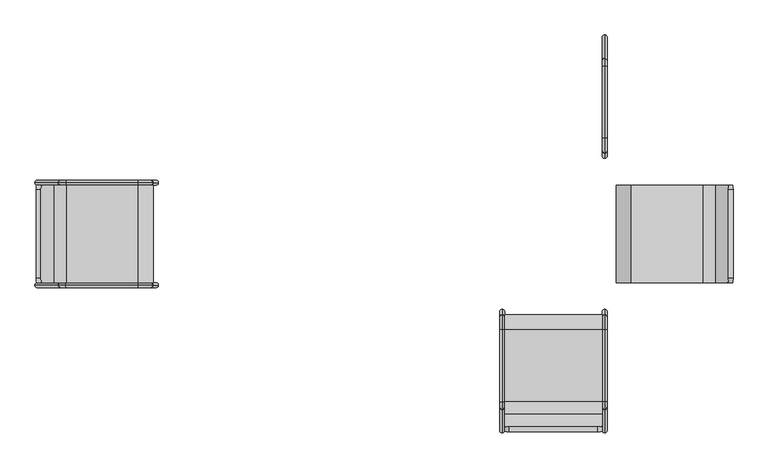
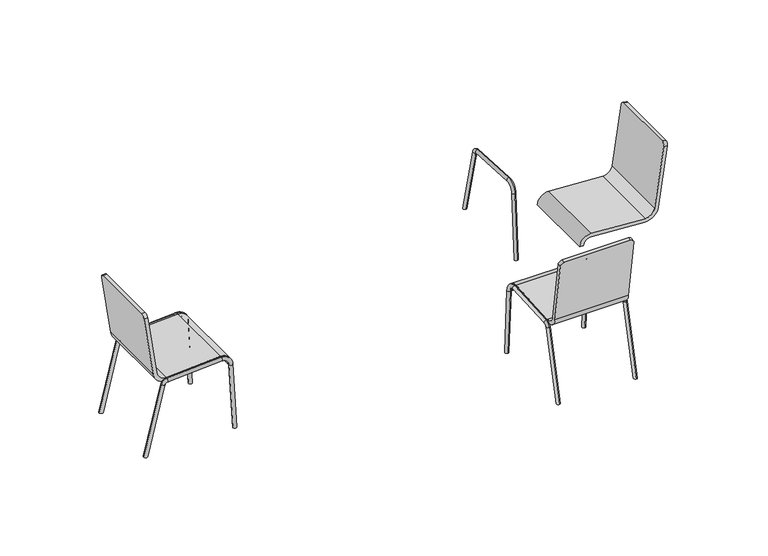
"""IFC4 building model written with IfcOpenShell, lengths in millimetres: furniture geometry."""

from ifc_helpers import new_model, si_unit, point, frame, origin, place, context, project, spatial, polyline, circle_curve, ellipse_curve, trimmed, source, transform, mapped, element, save
from ifc_brep_helpers import plane_surface, cylinder_surface, revolved_surface, advanced_brep


def furniture_b53a9923(model_context):
    return source(origin(), model_context, "Body", "AdvancedBrep", [
        advanced_brep(
        [(832.7255181, 202.5, 414.5657988), (885.0808804, 202.5, 457.0908917), (935.9370847, 202.5, 797.3777006), (955.717402, 202.5, 794.4215124), (904.8611977, 202.5, 454.1347035), (831.5636904, 202.5, 394.5995734), (535.5224482, 202.5, 411.8261096), (493.2663421, 202.5, 374.2173141), (473.3001167, 202.5, 375.3791418), (536.6842759, 202.5, 431.792335), (832.7255181, -202.5, 414.5657988), (536.6842759, -202.5, 431.792335), (473.3001167, -202.5, 375.3791418), (493.2663421, -202.5, 374.2173141), (535.5224482, -202.5, 411.8261096), (831.5636904, -202.5, 394.5995734), (904.8611977, -202.5, 454.1347035), (955.717402, -202.5, 794.4215124), (935.9370847, -202.5, 797.3777006), (885.0808804, -202.5, 457.0908917), (958.6735902, 182.5, 814.2018297), (958.6735902, -182.5, 814.2018297), (938.893273, 182.5, 817.1580179), (938.893273, -182.5, 817.1580179)],
        [
            (0, 1, circle_curve(frame((835.6300872, 202.5, 464.4813623), z_axis=(0.0, -1.0, 0.0), x_axis=(1.0, 0.0, 0.0)), 50.0)),
            (1, 2),
            (2, 3),
            (3, 4),
            (4, 5, circle_curve(frame((835.6300872, 202.5, 464.4813623), z_axis=(0.0, 1.0, 0.0), x_axis=(1.0, 0.0, 0.0)), 70.0)),
            (5, 6),
            (6, 7, circle_curve(frame((533.1987929, 202.5, 371.8936588), z_axis=(0.0, -1.0, 0.0), x_axis=(1.0, 0.0, 0.0)), 40.0)),
            (7, 8),
            (8, 9, circle_curve(frame((533.1987929, 202.5, 371.8936588), z_axis=(0.0, 1.0, 0.0), x_axis=(1.0, 0.0, 0.0)), 60.0)),
            (9, 0),
            (10, 11),
            (11, 12, circle_curve(frame((533.1987929, -202.5, 371.8936588), z_axis=(0.0, -1.0, 0.0), x_axis=(1.0, 0.0, 0.0)), 60.0)),
            (12, 13),
            (13, 14, circle_curve(frame((533.1987929, -202.5, 371.8936588), z_axis=(0.0, 1.0, 0.0), x_axis=(1.0, 0.0, 0.0)), 40.0)),
            (14, 15),
            (15, 16, circle_curve(frame((835.6300872, -202.5, 464.4813623), z_axis=(0.0, -1.0, 0.0), x_axis=(1.0, 0.0, 0.0)), 70.0)),
            (16, 17),
            (17, 18),
            (18, 19),
            (19, 10, circle_curve(frame((835.6300872, -202.5, 464.4813623), z_axis=(0.0, 1.0, 0.0), x_axis=(1.0, 0.0, 0.0)), 50.0)),
            (9, 11),
            (10, 0),
            (8, 12),
            (7, 13),
            (6, 14),
            (5, 15),
            (4, 16),
            (3, 20, circle_curve(frame((955.717402, 182.5, 794.4215124), z_axis=(0.9890158633619166, 0.0, -0.14780941112961252), x_axis=(0.0, -1.0, 0.0)), 20.0)),
            (20, 21),
            (21, 17, circle_curve(frame((955.717402, -182.5, 794.4215124), z_axis=(0.9890158633619166, 0.0, -0.14780941112961252), x_axis=(0.0, 1.0, 0.0)), 20.0)),
            (20, 22),
            (22, 23),
            (23, 21),
            (18, 23, circle_curve(frame((935.9370847, -182.5, 797.3777006), z_axis=(-0.9890158633619166, 0.0, 0.14780941112961252), x_axis=(0.0, 1.0, 0.0)), 20.0)),
            (22, 2, circle_curve(frame((935.9370847, 182.5, 797.3777006), z_axis=(-0.9890158633619166, 0.0, 0.14780941112961252), x_axis=(0.0, -1.0, 0.0)), 20.0)),
            (1, 19),
        ],
        [
            plane_surface(frame((538.9293412, 202.5, 431.6616954), z_axis=(0.0, 1.0000000000000002, 0.0), x_axis=(-0.9983112697039764, 0.0, 0.05809138302738736))),
            plane_surface(frame((538.9293412, -202.5, 431.6616954), z_axis=(0.0, -1.0000000000000002, 0.0), x_axis=(0.9983112697039764, 0.0, -0.05809138302738736))),
            plane_surface(frame((832.7255181, 202.5, 414.5657988), z_axis=(0.05809138302738736, 0.0, 0.9983112697039764), x_axis=(0.0, -1.0, 0.0))),
            cylinder_surface(frame((533.1987929, -202.5, 371.8936588), z_axis=(0.0, 1.0, 0.0), x_axis=(1.0, 0.0, 0.0)), 60.0),
            plane_surface(frame((473.3001167, 202.5, 375.3791418), z_axis=(-0.058091383027390926, 0.0, -0.9983112697039762), x_axis=(0.0, -1.0, 0.0))),
            revolved_surface(polyline([(573.1987929, -202.5, 371.8936588), (573.1987929, 202.5, 371.8936588)]), (533.1987929, -202.5, 371.8936588), (0.0, -1.0, 0.0)),
            plane_surface(frame((535.5224482, 202.5, 411.8261096), z_axis=(-0.05809138302738756, 0.0, -0.9983112697039763), x_axis=(0.0, -1.0, 0.0))),
            cylinder_surface(frame((835.6300872, -202.5, 464.4813623), z_axis=(0.0, 1.0, 0.0), x_axis=(1.0, 0.0, 0.0)), 70.0),
            plane_surface(frame((904.8611977, 202.5, 454.1347035), z_axis=(0.9890158633619166, 0.0, -0.1478094111296125), x_axis=(0.0, -1.0, 0.0))),
            plane_surface(frame((958.6735902, 202.5, 814.2018297), z_axis=(0.14780941112961524, 0.0, 0.9890158633619162), x_axis=(0.0, -1.0, 0.0))),
            plane_surface(frame((938.893273, 202.5, 817.1580179), z_axis=(-0.9890158633619166, 0.0, 0.14780941112961254), x_axis=(0.0, -1.0, 0.0))),
            revolved_surface(polyline([(885.6300872, -202.5, 464.4813623), (885.6300872, 202.5, 464.4813623)]), (835.6300872, -202.5, 464.4813623), (0.0, -1.0, 0.0)),
            cylinder_surface(frame((935.9370847, -182.5, 797.3777006), z_axis=(-0.9890158633619166, 0.0, 0.14780941112961252), x_axis=(0.0, 1.0, 0.0)), 20.0),
            cylinder_surface(frame((935.9370847, 182.5, 797.3777006), z_axis=(-0.9890158633619166, 0.0, 0.14780941112961252), x_axis=(0.0, -1.0, 0.0)), 20.0),
        ],
        [
            (0, [[1, 2, 3, 4, 5, 6, 7, 8, 9, 10]]),
            (1, [[11, 12, 13, 14, 15, 16, 17, 18, 19, 20]]),
            (2, [[21, -11, 22, -10]]),
            (3, [[23, -12, -21, -9]]),
            (4, [[24, -13, -23, -8]]),
            (5, [[25, -14, -24, -7]]),
            (6, [[26, -15, -25, -6]]),
            (7, [[27, -16, -26, -5]]),
            (8, [[-4, 28, 29, 30, -17, -27]]),
            (9, [[31, 32, 33, -29]]),
            (10, [[-19, 34, -32, 35, -2, 36]]),
            (11, [[-22, -20, -36, -1]]),
            (12, [[-30, -33, -34, -18]]),
            (13, [[-35, -31, -28, -3]]),
        ],
    ),
        advanced_brep(
        [(-1916.2585347, 212.5797007, 0.0), (-1936.8708073, 212.5797007, 0.0), (-1434.6031938, 222.5797007, 0.0), (-1434.6031938, 202.5797007, 0.0), (-1444.6201096, 212.5797007, 0.0), (-1820.7368981, 212.5797007, 383.1163586), (-1840.1428126, 212.5797007, 387.9547965), (-1807.053833, 212.5797007, 394.4621992), (-1808.2156606, 212.5797007, 414.4284246), (-1508.6517901, 212.5797007, 411.8261096), (-1509.8136178, 212.5797007, 431.792335), (-1466.395684, 212.5797007, 374.2173141), (-1446.4294586, 212.5797007, 375.3791418), (-1424.6200811, 212.5797007, 0.5809138)],
        [
            (0, 1, ellipse_curve(frame((-1926.564671, 212.5797007, 0.0), z_axis=(0.0, 0.0, -1.0), x_axis=(-1.0, 0.0, 0.0)), 10.3061363, 10.0)),
            (1, 0, ellipse_curve(frame((-1926.564671, 212.5797007, 0.0), z_axis=(0.0, 0.0, -1.0), x_axis=(-1.0, 0.0, 0.0)), 10.3061363, 10.0)),
            (2, 3),
            (3, 4, ellipse_curve(frame((-1434.6031938, 212.5797007, 0.0), z_axis=(0.0, 0.0, -1.0), x_axis=(-1.0, 0.0, 0.0)), 10.0169159, 10.0)),
            (4, 2, ellipse_curve(frame((-1434.6031938, 212.5797007, 0.0), z_axis=(0.0, 0.0, -1.0), x_axis=(-1.0, 0.0, 0.0)), 10.0169159, 10.0)),
            (5, 6, circle_curve(frame((-1830.4398554, 212.5797007, 385.5355776), z_axis=(-0.24192189559966623, 0.0, -0.9702957262759968), x_axis=(-0.9702957262759968, 0.0, 0.24192189559966623)), 10.0)),
            (6, 1),
            (0, 5),
            (6, 5, circle_curve(frame((-1830.4398554, 212.5797007, 385.5355776), z_axis=(-0.24192189559966623, 0.0, -0.9702957262759968), x_axis=(-0.9702957262759968, 0.0, 0.24192189559966623)), 10.0)),
            (5, 7, circle_curve(frame((-1806.1824622, 212.5797007, 379.4875302), z_axis=(0.0, 1.0, 0.0), x_axis=(-0.9702957262759969, 0.0, 0.2419218955996659)), 15.0)),
            (7, 8, circle_curve(frame((-1807.6347468, 212.5797007, 404.4453119), z_axis=(-0.998311269703977, 0.0, -0.058091383027376764), x_axis=(-0.058091383027376764, 0.0, 0.998311269703977)), 10.0)),
            (8, 6, circle_curve(frame((-1806.1824622, 212.5797007, 379.4875302), z_axis=(0.0, -1.0, 0.0), x_axis=(-0.9702957262759969, 0.0, 0.2419218955996659)), 35.0)),
            (8, 7, circle_curve(frame((-1807.6347468, 212.5797007, 404.4453119), z_axis=(-0.9983112697039765, 0.0, -0.05809138302738498), x_axis=(-0.05809138302738498, 0.0, 0.9983112697039765)), 10.0)),
            (7, 9),
            (9, 10, circle_curve(frame((-1509.232704, 212.5797007, 421.8092223), z_axis=(-0.9983112697039764, 0.0, -0.058091383027386895), x_axis=(-0.058091383027386895, 0.0, 0.9983112697039764)), 10.0)),
            (10, 8),
            (10, 9, circle_curve(frame((-1509.232704, 212.5797007, 421.8092223), z_axis=(-0.9983112697039764, 0.0, -0.058091383027386895), x_axis=(-0.058091383027386895, 0.0, 0.9983112697039764)), 10.0)),
            (9, 11, circle_curve(frame((-1506.3281348, 212.5797007, 371.8936588), z_axis=(0.0, 1.0, 0.0), x_axis=(-0.05809138302738633, 0.0, 0.9983112697039764)), 40.0)),
            (11, 12, circle_curve(frame((-1456.4125713, 212.5797007, 374.7982279), z_axis=(-0.058091383027391474, 0.0, 0.9983112697039761), x_axis=(0.9983112697039761, 0.0, 0.058091383027391474)), 10.0)),
            (12, 10, circle_curve(frame((-1506.3281348, 212.5797007, 371.8936588), z_axis=(0.0, -1.0, 0.0), x_axis=(-0.05809138302738633, 0.0, 0.9983112697039764)), 60.0)),
            (12, 11, circle_curve(frame((-1456.4125713, 212.5797007, 374.7982279), z_axis=(-0.05809138302739081, 0.0, 0.9983112697039762), x_axis=(0.9983112697039762, 0.0, 0.05809138302739081)), 10.0)),
            (2, 13, circle_curve(frame((-1434.6031938, 212.5797007, 0.0), z_axis=(0.058091383027392335, 0.0, -0.9983112697039761), x_axis=(0.9983112697039761, 0.0, 0.058091383027392335)), 10.0)),
            (13, 3, circle_curve(frame((-1434.6031938, 212.5797007, 0.0), z_axis=(0.058091383027392335, 0.0, -0.9983112697039761), x_axis=(0.9983112697039761, 0.0, 0.058091383027392335)), 10.0)),
            (11, 4),
            (13, 12),
        ],
        [
            plane_surface(frame((-1962.0110531, 250.0, 0.0), z_axis=(0.0, 0.0, -1.0), x_axis=(0.0, -1.0, 0.0))),
            cylinder_surface(frame((-1929.1748213, 212.5797007, -10.4687411), z_axis=(-0.24192189559966623, 0.0, -0.9702957262759968), x_axis=(-0.9702957262759968, 0.0, 0.24192189559966623)), 10.0),
            revolved_surface(trimmed(ellipse_curve(frame((-1830.4398554, 212.5797007, 385.5355776), z_axis=(-0.2419218955996659, 0.0, -0.9702957262759969), x_axis=(-0.9702957262759969, 0.0, 0.2419218955996659)), 10.0, 10.0), [point((-1820.7368981, 212.5797007, 383.1163586))], [point((-1840.1428126, 212.5797007, 387.9547965))], True, "CARTESIAN"), (-1806.1824622, 192.5797007, 379.4875302), (0.0, 1.0, 0.0)),
            revolved_surface(trimmed(ellipse_curve(frame((-1830.4398554, 212.5797007, 385.5355776), z_axis=(-0.2419218955996659, 0.0, -0.9702957262759969), x_axis=(-0.9702957262759969, 0.0, 0.2419218955996659)), 10.0, 10.0), [point((-1840.1428126, 212.5797007, 387.9547965))], [point((-1820.7368981, 212.5797007, 383.1163586))], True, "CARTESIAN"), (-1806.1824622, 192.5797007, 379.4875302), (0.0, 1.0, 0.0)),
            cylinder_surface(frame((-1807.6347468, 212.5797007, 404.4453119), z_axis=(-0.9983112697039764, 0.0, -0.058091383027386895), x_axis=(-0.058091383027386895, 0.0, 0.9983112697039764)), 10.0),
            revolved_surface(trimmed(ellipse_curve(frame((-1509.232704, 212.5797007, 421.8092223), z_axis=(-0.9983112697039764, 0.0, -0.05809138302738631), x_axis=(-0.05809138302738631, 0.0, 0.9983112697039764)), 10.0, 10.0), [point((-1508.6517901, 212.5797007, 411.8261096))], [point((-1509.8136178, 212.5797007, 431.792335))], True, "CARTESIAN"), (-1506.3281348, 192.5797007, 371.8936588), (0.0, 1.0, 0.0)),
            revolved_surface(trimmed(ellipse_curve(frame((-1509.232704, 212.5797007, 421.8092223), z_axis=(-0.9983112697039764, 0.0, -0.05809138302738631), x_axis=(-0.05809138302738631, 0.0, 0.9983112697039764)), 10.0, 10.0), [point((-1509.8136178, 212.5797007, 431.792335))], [point((-1508.6517901, 212.5797007, 411.8261096))], True, "CARTESIAN"), (-1506.3281348, 192.5797007, 371.8936588), (0.0, 1.0, 0.0)),
            plane_surface(frame((-1434.6031938, 192.5797007, 0.0), z_axis=(0.058091383027392335, 0.0, -0.9983112697039761), x_axis=(0.0, 1.0, 0.0))),
            cylinder_surface(frame((-1456.4125713, 212.5797007, 374.7982279), z_axis=(-0.058091383027392335, 0.0, 0.9983112697039761), x_axis=(0.9983112697039761, 0.0, 0.058091383027392335)), 10.0),
        ],
        [
            (0, [[1, 2]]),
            (0, [[3, 4, 5]]),
            (1, [[6, 7, -1, 8]]),
            (1, [[9, -8, -2, -7]]),
            (2, [[-6, 10, 11, 12]]),
            (3, [[-9, -12, 13, -10]]),
            (4, [[-11, 14, 15, 16]]),
            (4, [[-13, -16, 17, -14]]),
            (5, [[-15, 18, 19, 20]]),
            (6, [[-17, -20, 21, -18]]),
            (7, [[22, 23, -3]]),
            (8, [[-19, 24, -4, -23, 25]]),
            (8, [[-21, -25, -22, -5, -24]]),
        ],
    ),
        advanced_brep(
        [(-1434.6031938, -202.5797007, 0.0), (-1424.6200811, -212.5797007, 0.5809138), (-1434.6031938, -222.5797007, 0.0), (-1820.7368981, -212.5797007, 383.1163586), (-1840.1428126, -212.5797007, 387.9547965), (-1936.8708073, -212.5797007, 0.0), (-1916.2585347, -212.5797007, 0.0), (-1444.6201096, -212.5797007, 0.0), (-1808.2156606, -212.5797007, 414.4284246), (-1807.053833, -212.5797007, 394.4621992), (-1508.6517901, -212.5797007, 411.8261096), (-1509.8136178, -212.5797007, 431.792335), (-1466.395684, -212.5797007, 374.2173141), (-1446.4294586, -212.5797007, 375.3791418)],
        [
            (0, 1, circle_curve(frame((-1434.6031938, -212.5797007, 0.0), z_axis=(0.058091383027392335, 0.0, -0.9983112697039761), x_axis=(0.9983112697039761, 0.0, 0.058091383027392335)), 10.0)),
            (1, 2, circle_curve(frame((-1434.6031938, -212.5797007, 0.0), z_axis=(0.058091383027392335, 0.0, -0.9983112697039761), x_axis=(0.9983112697039761, 0.0, 0.058091383027392335)), 10.0)),
            (2, 0),
            (3, 4, circle_curve(frame((-1830.4398554, -212.5797007, 385.5355776), z_axis=(-0.24192189559966623, 0.0, -0.9702957262759968), x_axis=(-0.9702957262759968, 0.0, 0.24192189559966623)), 10.0)),
            (4, 5),
            (5, 6, ellipse_curve(frame((-1926.564671, -212.5797007, 0.0), z_axis=(0.0, 0.0, 1.0), x_axis=(-1.0, 0.0, 0.0)), 10.3061363, 10.0)),
            (6, 3),
            (4, 3, circle_curve(frame((-1830.4398554, -212.5797007, 385.5355776), z_axis=(-0.24192189559966623, 0.0, -0.9702957262759968), x_axis=(-0.9702957262759968, 0.0, 0.24192189559966623)), 10.0)),
            (6, 5, ellipse_curve(frame((-1926.564671, -212.5797007, 0.0), z_axis=(0.0, 0.0, 1.0), x_axis=(-1.0, 0.0, 0.0)), 10.3061363, 10.0)),
            (2, 7, ellipse_curve(frame((-1434.6031938, -212.5797007, 0.0), z_axis=(0.0, 0.0, -1.0), x_axis=(-1.0, 0.0, 0.0)), 10.0169159, 10.0)),
            (7, 0, ellipse_curve(frame((-1434.6031938, -212.5797007, 0.0), z_axis=(0.0, 0.0, -1.0), x_axis=(-1.0, 0.0, 0.0)), 10.0169159, 10.0)),
            (8, 9, circle_curve(frame((-1807.6347468, -212.5797007, 404.4453119), z_axis=(0.9983112697039764, 0.0, 0.058091383027386895), x_axis=(-0.058091383027386895, 0.0, 0.9983112697039764)), 10.0)),
            (9, 10),
            (10, 11, circle_curve(frame((-1509.232704, -212.5797007, 421.8092223), z_axis=(-0.9983112697039764, 0.0, -0.058091383027386895), x_axis=(-0.058091383027386895, 0.0, 0.9983112697039764)), 10.0)),
            (11, 8),
            (9, 8, circle_curve(frame((-1807.6347468, -212.5797007, 404.4453119), z_axis=(0.9983112697039764, 0.0, 0.058091383027386895), x_axis=(-0.058091383027386895, 0.0, 0.9983112697039764)), 10.0)),
            (11, 10, circle_curve(frame((-1509.232704, -212.5797007, 421.8092223), z_axis=(-0.9983112697039764, 0.0, -0.058091383027386895), x_axis=(-0.058091383027386895, 0.0, 0.9983112697039764)), 10.0)),
            (10, 12, circle_curve(frame((-1506.3281348, -212.5797007, 371.8936588), z_axis=(0.0, 1.0, 0.0), x_axis=(-0.05809138302738633, 0.0, 0.9983112697039764)), 40.0)),
            (12, 13, circle_curve(frame((-1456.4125713, -212.5797007, 374.7982279), z_axis=(-0.058091383027391474, 0.0, 0.9983112697039761), x_axis=(0.9983112697039761, 0.0, 0.058091383027391474)), 10.0)),
            (13, 11, circle_curve(frame((-1506.3281348, -212.5797007, 371.8936588), z_axis=(0.0, -1.0, 0.0), x_axis=(-0.05809138302738633, 0.0, 0.9983112697039764)), 60.0)),
            (13, 12, circle_curve(frame((-1456.4125713, -212.5797007, 374.7982279), z_axis=(-0.05809138302739081, 0.0, 0.9983112697039762), x_axis=(0.9983112697039762, 0.0, 0.05809138302739081)), 10.0)),
            (12, 7),
            (1, 13),
            (3, 9, circle_curve(frame((-1806.1824622, -212.5797007, 379.4875302), z_axis=(0.0, 1.0, 0.0), x_axis=(-0.9702957262759969, 0.0, 0.2419218955996659)), 15.0)),
            (8, 4, circle_curve(frame((-1806.1824622, -212.5797007, 379.4875302), z_axis=(0.0, -1.0, 0.0), x_axis=(-0.9702957262759969, 0.0, 0.2419218955996659)), 35.0)),
        ],
        [
            plane_surface(frame((-1434.6031938, -192.5797007, 0.0), z_axis=(0.058091383027392335, 0.0, -0.9983112697039761), x_axis=(0.0, -1.0, 0.0))),
            cylinder_surface(frame((-1929.1748213, -212.5797007, -10.4687411), z_axis=(-0.24192189559966623, 0.0, -0.9702957262759968), x_axis=(-0.9702957262759968, 0.0, 0.24192189559966623)), 10.0),
            plane_surface(frame((-1962.0110531, 250.0, 0.0), z_axis=(0.0, 0.0, -1.0), x_axis=(0.0, -1.0, 0.0))),
            cylinder_surface(frame((-1807.6347468, -212.5797007, 404.4453119), z_axis=(-0.9983112697039764, 0.0, -0.058091383027386895), x_axis=(-0.058091383027386895, 0.0, 0.9983112697039764)), 10.0),
            revolved_surface(trimmed(ellipse_curve(frame((-1509.232704, -212.5797007, 421.8092223), z_axis=(-0.9983112697039764, 0.0, -0.05809138302738631), x_axis=(-0.05809138302738631, 0.0, 0.9983112697039764)), 10.0, 10.0), [point((-1508.6517901, -212.5797007, 411.8261096))], [point((-1509.8136178, -212.5797007, 431.792335))], True, "CARTESIAN"), (-1506.3281348, -192.5797007, 371.8936588), (0.0, 1.0, 0.0)),
            revolved_surface(trimmed(ellipse_curve(frame((-1509.232704, -212.5797007, 421.8092223), z_axis=(-0.9983112697039764, 0.0, -0.05809138302738631), x_axis=(-0.05809138302738631, 0.0, 0.9983112697039764)), 10.0, 10.0), [point((-1509.8136178, -212.5797007, 431.792335))], [point((-1508.6517901, -212.5797007, 411.8261096))], True, "CARTESIAN"), (-1506.3281348, -192.5797007, 371.8936588), (0.0, 1.0, 0.0)),
            cylinder_surface(frame((-1456.4125713, -212.5797007, 374.7982279), z_axis=(-0.058091383027392335, 0.0, 0.9983112697039761), x_axis=(0.9983112697039761, 0.0, 0.058091383027392335)), 10.0),
            revolved_surface(trimmed(ellipse_curve(frame((-1830.4398554, -212.5797007, 385.5355776), z_axis=(-0.2419218955996659, 0.0, -0.9702957262759969), x_axis=(-0.9702957262759969, 0.0, 0.2419218955996659)), 10.0, 10.0), [point((-1820.7368981, -212.5797007, 383.1163586))], [point((-1840.1428126, -212.5797007, 387.9547965))], True, "CARTESIAN"), (-1806.1824622, -192.5797007, 379.4875302), (0.0, 1.0, 0.0)),
            revolved_surface(trimmed(ellipse_curve(frame((-1830.4398554, -212.5797007, 385.5355776), z_axis=(-0.2419218955996659, 0.0, -0.9702957262759969), x_axis=(-0.9702957262759969, 0.0, 0.2419218955996659)), 10.0, 10.0), [point((-1840.1428126, -212.5797007, 387.9547965))], [point((-1820.7368981, -212.5797007, 383.1163586))], True, "CARTESIAN"), (-1806.1824622, -192.5797007, 379.4875302), (0.0, 1.0, 0.0)),
        ],
        [
            (0, [[1, 2, 3]]),
            (1, [[4, 5, 6, 7]]),
            (1, [[8, -7, 9, -5]]),
            (2, [[-3, 10, 11]]),
            (2, [[-6, -9]]),
            (3, [[12, 13, 14, 15]]),
            (3, [[16, -15, 17, -13]]),
            (4, [[-14, 18, 19, 20]]),
            (5, [[-17, -20, 21, -18]]),
            (6, [[-19, 22, -10, -2, 23]]),
            (6, [[-21, -23, -1, -11, -22]]),
            (7, [[-4, 24, -12, 25]]),
            (8, [[-8, -25, -16, -24]]),
        ],
    ),
        advanced_brep(
        [(-1805.85486, 202.5, 414.5657988), (-1509.8136178, 202.5, 431.792335), (-1446.4294586, 202.5, 375.3791418), (-1466.395684, 202.5, 374.2173141), (-1508.6517901, 202.5, 411.8261096), (-1804.6930323, 202.5, 394.5995734), (-1877.9905396, 202.5, 454.1347035), (-1928.8467439, 202.5, 794.4215124), (-1909.0664267, 202.5, 797.3777006), (-1858.2102223, 202.5, 457.0908917), (-1805.85486, -202.5, 414.5657988), (-1858.2102223, -202.5, 457.0908917), (-1909.0664267, -202.5, 797.3777006), (-1928.8467439, -202.5, 794.4215124), (-1877.9905396, -202.5, 454.1347035), (-1804.6930323, -202.5, 394.5995734), (-1508.6517901, -202.5, 411.8261096), (-1466.395684, -202.5, 374.2173141), (-1446.4294586, -202.5, 375.3791418), (-1509.8136178, -202.5, 431.792335), (-1931.8029322, -182.5, 814.2018297), (-1931.8029322, 182.5, 814.2018297), (-1912.0226149, -182.5, 817.1580179), (-1912.0226149, 182.5, 817.1580179)],
        [
            (0, 1),
            (1, 2, circle_curve(frame((-1506.3281348, 202.5, 371.8936588), z_axis=(0.0, 1.0, 0.0), x_axis=(-1.0, 0.0, 0.0)), 60.0)),
            (2, 3),
            (3, 4, circle_curve(frame((-1506.3281348, 202.5, 371.8936588), z_axis=(0.0, -1.0, 0.0), x_axis=(-1.0, 0.0, 0.0)), 40.0)),
            (4, 5),
            (5, 6, circle_curve(frame((-1808.7594292, 202.5, 464.4813623), z_axis=(0.0, 1.0, 0.0), x_axis=(-1.0, 0.0, 0.0)), 70.0)),
            (6, 7),
            (7, 8),
            (8, 9),
            (9, 0, circle_curve(frame((-1808.7594292, 202.5, 464.4813623), z_axis=(0.0, -1.0, 0.0), x_axis=(-1.0, 0.0, 0.0)), 50.0)),
            (10, 11, circle_curve(frame((-1808.7594292, -202.5, 464.4813623), z_axis=(0.0, 1.0, 0.0), x_axis=(-1.0, 0.0, 0.0)), 50.0)),
            (11, 12),
            (12, 13),
            (13, 14),
            (14, 15, circle_curve(frame((-1808.7594292, -202.5, 464.4813623), z_axis=(0.0, -1.0, 0.0), x_axis=(-1.0, 0.0, 0.0)), 70.0)),
            (15, 16),
            (16, 17, circle_curve(frame((-1506.3281348, -202.5, 371.8936588), z_axis=(0.0, 1.0, 0.0), x_axis=(-1.0, 0.0, 0.0)), 40.0)),
            (17, 18),
            (18, 19, circle_curve(frame((-1506.3281348, -202.5, 371.8936588), z_axis=(0.0, -1.0, 0.0), x_axis=(-1.0, 0.0, 0.0)), 60.0)),
            (19, 10),
            (0, 10),
            (19, 1),
            (18, 2),
            (17, 3),
            (16, 4),
            (15, 5),
            (14, 6),
            (13, 20, circle_curve(frame((-1928.8467439, -182.5, 794.4215124), z_axis=(-0.9890158633619166, 0.0, -0.14780941112961252), x_axis=(0.0, 1.0, 0.0)), 20.0)),
            (20, 21),
            (21, 7, circle_curve(frame((-1928.8467439, 182.5, 794.4215124), z_axis=(-0.9890158633619166, 0.0, -0.14780941112961252), x_axis=(0.0, -1.0, 0.0)), 20.0)),
            (20, 22),
            (22, 23),
            (23, 21),
            (11, 9),
            (8, 23, circle_curve(frame((-1909.0664267, 182.5, 797.3777006), z_axis=(0.9890158633619166, 0.0, 0.14780941112961252), x_axis=(0.0, -1.0, 0.0)), 20.0)),
            (22, 12, circle_curve(frame((-1909.0664267, -182.5, 797.3777006), z_axis=(0.9890158633619166, 0.0, 0.14780941112961252), x_axis=(0.0, 1.0, 0.0)), 20.0)),
        ],
        [
            plane_surface(frame((-1512.0586831, 202.5, 431.6616954), z_axis=(0.0, 1.0000000000000002, 0.0), x_axis=(0.9983112697039764, 0.0, 0.05809138302738736))),
            plane_surface(frame((-1512.0586831, -202.5, 431.6616954), z_axis=(0.0, -1.0000000000000002, 0.0), x_axis=(-0.9983112697039764, 0.0, -0.05809138302738736))),
            plane_surface(frame((-1805.85486, 202.5, 414.5657988), z_axis=(-0.05809138302738736, 0.0, 0.9983112697039764), x_axis=(0.0, -1.0, 0.0))),
            cylinder_surface(frame((-1506.3281348, -202.5, 371.8936588), z_axis=(0.0, 1.0, 0.0), x_axis=(-1.0, 0.0, 0.0)), 60.0),
            plane_surface(frame((-1446.4294586, 202.5, 375.3791418), z_axis=(0.058091383027390926, 0.0, -0.9983112697039762), x_axis=(0.0, -1.0, 0.0))),
            revolved_surface(polyline([(-1546.3281348, -202.5, 371.8936588), (-1546.3281348, 202.5, 371.8936588)]), (-1506.3281348, -202.5, 371.8936588), (0.0, -1.0, 0.0)),
            plane_surface(frame((-1508.6517901, 202.5, 411.8261096), z_axis=(0.05809138302738756, 0.0, -0.9983112697039763), x_axis=(0.0, -1.0, 0.0))),
            cylinder_surface(frame((-1808.7594292, -202.5, 464.4813623), z_axis=(0.0, 1.0, 0.0), x_axis=(-1.0, 0.0, 0.0)), 70.0),
            plane_surface(frame((-1877.9905396, 202.5, 454.1347035), z_axis=(-0.9890158633619166, 0.0, -0.1478094111296125), x_axis=(0.0, -1.0, 0.0))),
            plane_surface(frame((-1931.8029322, 202.5, 814.2018297), z_axis=(-0.14780941112961524, 0.0, 0.9890158633619162), x_axis=(0.0, -1.0, 0.0))),
            plane_surface(frame((-1912.0226149, 202.5, 817.1580179), z_axis=(0.9890158633619166, 0.0, 0.14780941112961254), x_axis=(0.0, -1.0, 0.0))),
            revolved_surface(polyline([(-1858.7594292, -202.5, 464.4813623), (-1858.7594292, 202.5, 464.4813623)]), (-1808.7594292, -202.5, 464.4813623), (0.0, -1.0, 0.0)),
            cylinder_surface(frame((-1909.0664267, -182.5, 797.3777006), z_axis=(0.9890158633619166, 0.0, 0.14780941112961252), x_axis=(0.0, 1.0, 0.0)), 20.0),
            cylinder_surface(frame((-1909.0664267, 182.5, 797.3777006), z_axis=(0.9890158633619166, 0.0, 0.14780941112961252), x_axis=(0.0, -1.0, 0.0)), 20.0),
        ],
        [
            (0, [[1, 2, 3, 4, 5, 6, 7, 8, 9, 10]]),
            (1, [[11, 12, 13, 14, 15, 16, 17, 18, 19, 20]]),
            (2, [[-1, 21, -20, 22]]),
            (3, [[-2, -22, -19, 23]]),
            (4, [[-3, -23, -18, 24]]),
            (5, [[-4, -24, -17, 25]]),
            (6, [[-5, -25, -16, 26]]),
            (7, [[-6, -26, -15, 27]]),
            (8, [[-27, -14, 28, 29, 30, -7]]),
            (9, [[-29, 31, 32, 33]]),
            (10, [[34, -9, 35, -32, 36, -12]]),
            (11, [[-10, -34, -11, -21]]),
            (12, [[-13, -36, -31, -28]]),
            (13, [[-8, -30, -33, -35]]),
        ],
    ),
        advanced_brep(
        [(426.0150298, -804.6938637, 0.0), (426.0150298, -825.3061363, 0.0), (436.0150298, -323.0385228, 0.0), (426.0150298, -333.0554387, 0.0), (416.0150298, -323.0385228, 0.0), (426.0150298, -709.1722272, 383.1163586), (426.0150298, -728.5781417, 387.9547965), (426.0150298, -696.6509897, 414.4284246), (426.0150298, -695.489162, 394.4621992), (426.0150298, -398.2489468, 431.792335), (426.0150298, -397.0871192, 411.8261096), (426.0150298, -334.8647877, 375.3791418), (426.0150298, -354.8310131, 374.2173141), (426.0150298, -313.0554101, 0.5809138)],
        [
            (0, 1, ellipse_curve(frame((426.0150298, -815.0, 0.0), z_axis=(0.0, 0.0, -1.0), x_axis=(0.0, -1.0, 0.0)), 10.3061363, 10.0)),
            (1, 0, ellipse_curve(frame((426.0150298, -815.0, 0.0), z_axis=(0.0, 0.0, -1.0), x_axis=(0.0, -1.0, 0.0)), 10.3061363, 10.0)),
            (2, 3, ellipse_curve(frame((426.0150298, -323.0385228, 0.0), z_axis=(0.0, 0.0, -1.0), x_axis=(0.0, -1.0, 0.0)), 10.0169159, 10.0)),
            (3, 4, ellipse_curve(frame((426.0150298, -323.0385228, 0.0), z_axis=(0.0, 0.0, -1.0), x_axis=(0.0, -1.0, 0.0)), 10.0169159, 10.0)),
            (4, 2),
            (5, 0),
            (1, 6),
            (6, 5, circle_curve(frame((426.0150298, -718.8751844, 385.5355776), z_axis=(0.0, -0.24192189559966623, -0.9702957262759968), x_axis=(0.0, -0.9702957262759968, 0.24192189559966623)), 10.0)),
            (5, 6, circle_curve(frame((426.0150298, -718.8751844, 385.5355776), z_axis=(0.0, -0.24192189559966623, -0.9702957262759968), x_axis=(0.0, -0.9702957262759968, 0.24192189559966623)), 10.0)),
            (6, 7, circle_curve(frame((426.0150298, -694.6177913, 379.4875302), z_axis=(-1.0, 0.0, 0.0), x_axis=(0.0, -0.9702957262759969, 0.2419218955996659)), 35.0)),
            (7, 8, circle_curve(frame((426.0150298, -696.0700758, 404.4453119), z_axis=(0.0, -0.9983112697039765, -0.05809138302738456), x_axis=(0.0, -0.05809138302738456, 0.9983112697039765)), 10.0)),
            (8, 5, circle_curve(frame((426.0150298, -694.6177913, 379.4875302), z_axis=(1.0, 0.0, 0.0), x_axis=(0.0, -0.9702957262759969, 0.2419218955996659)), 15.0)),
            (8, 7, circle_curve(frame((426.0150298, -696.0700758, 404.4453119), z_axis=(0.0, -0.998311269703977, -0.05809138302737549), x_axis=(0.0, -0.05809138302737549, 0.998311269703977)), 10.0)),
            (7, 9),
            (9, 10, circle_curve(frame((426.0150298, -397.668033, 421.8092223), z_axis=(0.0, -0.9983112697039764, -0.058091383027386895), x_axis=(0.0, -0.058091383027386895, 0.9983112697039764)), 10.0)),
            (10, 8),
            (10, 9, circle_curve(frame((426.0150298, -397.668033, 421.8092223), z_axis=(0.0, -0.9983112697039764, -0.058091383027386895), x_axis=(0.0, -0.058091383027386895, 0.9983112697039764)), 10.0)),
            (9, 11, circle_curve(frame((426.0150298, -394.7634639, 371.8936588), z_axis=(-1.0, 0.0, 0.0), x_axis=(0.0, -0.05809138302738633, 0.9983112697039764)), 60.0)),
            (11, 12, circle_curve(frame((426.0150298, -344.8479004, 374.7982279), z_axis=(0.0, -0.05809138302739081, 0.9983112697039762), x_axis=(0.0, 0.9983112697039762, 0.05809138302739081)), 10.0)),
            (12, 10, circle_curve(frame((426.0150298, -394.7634639, 371.8936588), z_axis=(1.0, 0.0, 0.0), x_axis=(0.0, -0.05809138302738633, 0.9983112697039764)), 40.0)),
            (12, 11, circle_curve(frame((426.0150298, -344.8479004, 374.7982279), z_axis=(0.0, -0.05809138302739125, 0.9983112697039761), x_axis=(0.0, 0.9983112697039761, 0.05809138302739125)), 10.0)),
            (4, 13, circle_curve(frame((426.0150298, -323.0385228, 0.0), z_axis=(0.0, 0.058091383027392335, -0.9983112697039761), x_axis=(0.0, 0.9983112697039761, 0.058091383027392335)), 10.0)),
            (13, 2, circle_curve(frame((426.0150298, -323.0385228, 0.0), z_axis=(0.0, 0.058091383027392335, -0.9983112697039761), x_axis=(0.0, 0.9983112697039761, 0.058091383027392335)), 10.0)),
            (11, 13),
            (3, 12),
        ],
        [
            plane_surface(frame((463.435329, -850.4463822, 0.0), z_axis=(0.0, 0.0, -1.0), x_axis=(-1.0, 0.0, 0.0))),
            cylinder_surface(frame((426.0150298, -817.6101503, -10.4687411), z_axis=(0.0, -0.24192189559966623, -0.9702957262759968), x_axis=(0.0, -0.9702957262759968, 0.24192189559966623)), 10.0),
            revolved_surface(trimmed(ellipse_curve(frame((426.0150298, -718.8751844, 385.5355776), z_axis=(0.0, 0.2419218955996659, 0.9702957262759969), x_axis=(0.0, -0.9702957262759969, 0.2419218955996659)), 10.0, 10.0), [point((426.0150298, -709.1722272, 383.1163586))], [point((426.0150298, -728.5781417, 387.9547965))], True, "CARTESIAN"), (406.0150298, -694.6177913, 379.4875302), (1.0, 0.0, 0.0)),
            revolved_surface(trimmed(ellipse_curve(frame((426.0150298, -718.8751844, 385.5355776), z_axis=(0.0, 0.2419218955996659, 0.9702957262759969), x_axis=(0.0, -0.9702957262759969, 0.2419218955996659)), 10.0, 10.0), [point((426.0150298, -728.5781417, 387.9547965))], [point((426.0150298, -709.1722272, 383.1163586))], True, "CARTESIAN"), (406.0150298, -694.6177913, 379.4875302), (1.0, 0.0, 0.0)),
            cylinder_surface(frame((426.0150298, -696.0700758, 404.4453119), z_axis=(0.0, -0.9983112697039764, -0.058091383027386895), x_axis=(0.0, -0.058091383027386895, 0.9983112697039764)), 10.0),
            revolved_surface(trimmed(ellipse_curve(frame((426.0150298, -397.668033, 421.8092223), z_axis=(0.0, 0.9983112697039764, 0.05809138302738631), x_axis=(0.0, -0.05809138302738631, 0.9983112697039764)), 10.0, 10.0), [point((426.0150298, -397.0871192, 411.8261096))], [point((426.0150298, -398.2489468, 431.792335))], True, "CARTESIAN"), (406.0150298, -394.7634639, 371.8936588), (1.0, 0.0, 0.0)),
            revolved_surface(trimmed(ellipse_curve(frame((426.0150298, -397.668033, 421.8092223), z_axis=(0.0, 0.9983112697039764, 0.05809138302738631), x_axis=(0.0, -0.05809138302738631, 0.9983112697039764)), 10.0, 10.0), [point((426.0150298, -398.2489468, 431.792335))], [point((426.0150298, -397.0871192, 411.8261096))], True, "CARTESIAN"), (406.0150298, -394.7634639, 371.8936588), (1.0, 0.0, 0.0)),
            plane_surface(frame((406.0150298, -323.0385228, 0.0), z_axis=(0.0, 0.058091383027392335, -0.9983112697039761), x_axis=(1.0, 0.0, 0.0))),
            cylinder_surface(frame((426.0150298, -344.8479004, 374.7982279), z_axis=(0.0, -0.058091383027392335, 0.9983112697039761), x_axis=(0.0, 0.9983112697039761, 0.058091383027392335)), 10.0),
        ],
        [
            (0, [[1, 2]]),
            (0, [[3, 4, 5]]),
            (1, [[6, -2, 7, 8]]),
            (1, [[-7, -1, -6, 9]]),
            (2, [[10, 11, 12, -8]]),
            (3, [[-12, 13, -10, -9]]),
            (4, [[14, 15, 16, -11]]),
            (4, [[-16, 17, -14, -13]]),
            (5, [[18, 19, 20, -15]]),
            (6, [[-20, 21, -18, -17]]),
            (7, [[-5, 22, 23]]),
            (8, [[24, -22, -4, 25, -19]]),
            (8, [[-25, -3, -23, -24, -21]]),
        ],
    ),
        advanced_brep(
        [(10.8556283, -323.0385228, 0.0), (-9.1443717, -323.0385228, 0.0), (0.8556283, -313.0554101, 0.5809138), (0.8556283, -709.1722272, 383.1163586), (0.8556283, -804.6938637, 0.0), (0.8556283, -825.3061363, 0.0), (0.8556283, -728.5781417, 387.9547965), (0.8556283, -333.0554387, 0.0), (0.8556283, -696.6509897, 414.4284246), (0.8556283, -398.2489468, 431.792335), (0.8556283, -397.0871192, 411.8261096), (0.8556283, -695.489162, 394.4621992), (0.8556283, -334.8647877, 375.3791418), (0.8556283, -354.8310131, 374.2173141)],
        [
            (0, 1),
            (1, 2, circle_curve(frame((0.8556283, -323.0385228, 0.0), z_axis=(0.0, 0.058091383027392335, -0.9983112697039761), x_axis=(0.0, 0.9983112697039761, 0.058091383027392335)), 10.0)),
            (2, 0, circle_curve(frame((0.8556283, -323.0385228, 0.0), z_axis=(0.0, 0.058091383027392335, -0.9983112697039761), x_axis=(0.0, 0.9983112697039761, 0.058091383027392335)), 10.0)),
            (3, 4),
            (4, 5, ellipse_curve(frame((0.8556283, -815.0, 0.0), z_axis=(0.0, 0.0, 1.0), x_axis=(0.0, -1.0, 0.0)), 10.3061363, 10.0)),
            (5, 6),
            (6, 3, circle_curve(frame((0.8556283, -718.8751844, 385.5355776), z_axis=(0.0, -0.24192189559966623, -0.9702957262759968), x_axis=(0.0, -0.9702957262759968, 0.24192189559966623)), 10.0)),
            (5, 4, ellipse_curve(frame((0.8556283, -815.0, 0.0), z_axis=(0.0, 0.0, 1.0), x_axis=(0.0, -1.0, 0.0)), 10.3061363, 10.0)),
            (3, 6, circle_curve(frame((0.8556283, -718.8751844, 385.5355776), z_axis=(0.0, -0.24192189559966623, -0.9702957262759968), x_axis=(0.0, -0.9702957262759968, 0.24192189559966623)), 10.0)),
            (0, 7, ellipse_curve(frame((0.8556283, -323.0385228, 0.0), z_axis=(0.0, 0.0, -1.0), x_axis=(0.0, -1.0, 0.0)), 10.0169159, 10.0)),
            (7, 1, ellipse_curve(frame((0.8556283, -323.0385228, 0.0), z_axis=(0.0, 0.0, -1.0), x_axis=(0.0, -1.0, 0.0)), 10.0169159, 10.0)),
            (8, 9),
            (9, 10, circle_curve(frame((0.8556283, -397.668033, 421.8092223), z_axis=(0.0, -0.9983112697039764, -0.058091383027386895), x_axis=(0.0, -0.058091383027386895, 0.9983112697039764)), 10.0)),
            (10, 11),
            (11, 8, circle_curve(frame((0.8556283, -696.0700758, 404.4453119), z_axis=(0.0, 0.9983112697039764, 0.058091383027386895), x_axis=(0.0, -0.058091383027386895, 0.9983112697039764)), 10.0)),
            (10, 9, circle_curve(frame((0.8556283, -397.668033, 421.8092223), z_axis=(0.0, -0.9983112697039764, -0.058091383027386895), x_axis=(0.0, -0.058091383027386895, 0.9983112697039764)), 10.0)),
            (8, 11, circle_curve(frame((0.8556283, -696.0700758, 404.4453119), z_axis=(0.0, 0.9983112697039764, 0.058091383027386895), x_axis=(0.0, -0.058091383027386895, 0.9983112697039764)), 10.0)),
            (9, 12, circle_curve(frame((0.8556283, -394.7634639, 371.8936588), z_axis=(-1.0, 0.0, 0.0), x_axis=(0.0, -0.05809138302738633, 0.9983112697039764)), 60.0)),
            (12, 13, circle_curve(frame((0.8556283, -344.8479004, 374.7982279), z_axis=(0.0, -0.058091383027391474, 0.9983112697039761), x_axis=(0.0, 0.9983112697039761, 0.058091383027391474)), 10.0)),
            (13, 10, circle_curve(frame((0.8556283, -394.7634639, 371.8936588), z_axis=(1.0, 0.0, 0.0), x_axis=(0.0, -0.05809138302738633, 0.9983112697039764)), 40.0)),
            (13, 12, circle_curve(frame((0.8556283, -344.8479004, 374.7982279), z_axis=(0.0, -0.05809138302739081, 0.9983112697039762), x_axis=(0.0, 0.9983112697039762, 0.05809138302739081)), 10.0)),
            (12, 2),
            (7, 13),
            (6, 8, circle_curve(frame((0.8556283, -694.6177913, 379.4875302), z_axis=(-1.0, 0.0, 0.0), x_axis=(0.0, -0.9702957262759969, 0.2419218955996659)), 35.0)),
            (11, 3, circle_curve(frame((0.8556283, -694.6177913, 379.4875302), z_axis=(1.0, 0.0, 0.0), x_axis=(0.0, -0.9702957262759969, 0.2419218955996659)), 15.0)),
        ],
        [
            plane_surface(frame((20.8556283, -323.0385228, 0.0), z_axis=(0.0, 0.058091383027392335, -0.9983112697039761), x_axis=(-1.0, 0.0, 0.0))),
            cylinder_surface(frame((0.8556283, -817.6101503, -10.4687411), z_axis=(0.0, -0.24192189559966623, -0.9702957262759968), x_axis=(0.0, -0.9702957262759968, 0.24192189559966623)), 10.0),
            plane_surface(frame((463.435329, -850.4463822, 0.0), z_axis=(0.0, 0.0, -1.0), x_axis=(-1.0, 0.0, 0.0))),
            cylinder_surface(frame((0.8556283, -696.0700758, 404.4453119), z_axis=(0.0, -0.9983112697039764, -0.058091383027386895), x_axis=(0.0, -0.058091383027386895, 0.9983112697039764)), 10.0),
            revolved_surface(trimmed(ellipse_curve(frame((0.8556283, -397.668033, 421.8092223), z_axis=(0.0, 0.9983112697039764, 0.05809138302738631), x_axis=(0.0, -0.05809138302738631, 0.9983112697039764)), 10.0, 10.0), [point((0.8556283, -397.0871192, 411.8261096))], [point((0.8556283, -398.2489468, 431.792335))], True, "CARTESIAN"), (20.8556283, -394.7634639, 371.8936588), (1.0, 0.0, 0.0)),
            revolved_surface(trimmed(ellipse_curve(frame((0.8556283, -397.668033, 421.8092223), z_axis=(0.0, 0.9983112697039764, 0.05809138302738631), x_axis=(0.0, -0.05809138302738631, 0.9983112697039764)), 10.0, 10.0), [point((0.8556283, -398.2489468, 431.792335))], [point((0.8556283, -397.0871192, 411.8261096))], True, "CARTESIAN"), (20.8556283, -394.7634639, 371.8936588), (1.0, 0.0, 0.0)),
            cylinder_surface(frame((0.8556283, -344.8479004, 374.7982279), z_axis=(0.0, -0.058091383027392335, 0.9983112697039761), x_axis=(0.0, 0.9983112697039761, 0.058091383027392335)), 10.0),
            revolved_surface(trimmed(ellipse_curve(frame((0.8556283, -718.8751844, 385.5355776), z_axis=(0.0, 0.2419218955996659, 0.9702957262759969), x_axis=(0.0, -0.9702957262759969, 0.2419218955996659)), 10.0, 10.0), [point((0.8556283, -709.1722272, 383.1163586))], [point((0.8556283, -728.5781417, 387.9547965))], True, "CARTESIAN"), (20.8556283, -694.6177913, 379.4875302), (1.0, 0.0, 0.0)),
            revolved_surface(trimmed(ellipse_curve(frame((0.8556283, -718.8751844, 385.5355776), z_axis=(0.0, 0.2419218955996659, 0.9702957262759969), x_axis=(0.0, -0.9702957262759969, 0.2419218955996659)), 10.0, 10.0), [point((0.8556283, -728.5781417, 387.9547965))], [point((0.8556283, -709.1722272, 383.1163586))], True, "CARTESIAN"), (20.8556283, -694.6177913, 379.4875302), (1.0, 0.0, 0.0)),
        ],
        [
            (0, [[1, 2, 3]]),
            (1, [[4, 5, 6, 7]]),
            (1, [[-6, 8, -4, 9]]),
            (2, [[-8, -5]]),
            (2, [[10, 11, -1]]),
            (3, [[12, 13, 14, 15]]),
            (3, [[-14, 16, -12, 17]]),
            (4, [[18, 19, 20, -13]]),
            (5, [[-20, 21, -18, -16]]),
            (6, [[22, -2, -11, 23, -19]]),
            (6, [[-23, -10, -3, -22, -21]]),
            (7, [[24, -15, 25, -7]]),
            (8, [[-25, -17, -24, -9]]),
        ],
    ),
        advanced_brep(
        [(415.935329, -694.2901891, 414.5657988), (415.935329, -746.6455514, 457.0908917), (415.935329, -797.5017557, 797.3777006), (415.935329, -817.282073, 794.4215124), (415.935329, -766.4258686, 454.1347035), (415.935329, -693.1283614, 394.5995734), (415.935329, -397.0871192, 411.8261096), (415.935329, -354.8310131, 374.2173141), (415.935329, -334.8647877, 375.3791418), (415.935329, -398.2489468, 431.792335), (10.935329, -694.2901891, 414.5657988), (10.935329, -398.2489468, 431.792335), (10.935329, -334.8647877, 375.3791418), (10.935329, -354.8310131, 374.2173141), (10.935329, -397.0871192, 411.8261096), (10.935329, -693.1283614, 394.5995734), (10.935329, -766.4258686, 454.1347035), (10.935329, -817.282073, 794.4215124), (10.935329, -797.5017557, 797.3777006), (10.935329, -746.6455514, 457.0908917), (395.935329, -820.2382612, 814.2018297), (30.935329, -820.2382612, 814.2018297), (395.935329, -800.4579439, 817.1580179), (30.935329, -800.4579439, 817.1580179)],
        [
            (0, 1, circle_curve(frame((415.935329, -697.1947582, 464.4813623), z_axis=(-1.0, 0.0, 0.0), x_axis=(0.0, -1.0, 0.0)), 50.0)),
            (1, 2),
            (2, 3),
            (3, 4),
            (4, 5, circle_curve(frame((415.935329, -697.1947582, 464.4813623), z_axis=(1.0, 0.0, 0.0), x_axis=(0.0, -1.0, 0.0)), 70.0)),
            (5, 6),
            (6, 7, circle_curve(frame((415.935329, -394.7634639, 371.8936588), z_axis=(-1.0, 0.0, 0.0), x_axis=(0.0, -1.0, 0.0)), 40.0)),
            (7, 8),
            (8, 9, circle_curve(frame((415.935329, -394.7634639, 371.8936588), z_axis=(1.0, 0.0, 0.0), x_axis=(0.0, -1.0, 0.0)), 60.0)),
            (9, 0),
            (10, 11),
            (11, 12, circle_curve(frame((10.935329, -394.7634639, 371.8936588), z_axis=(-1.0, 0.0, 0.0), x_axis=(0.0, -1.0, 0.0)), 60.0)),
            (12, 13),
            (13, 14, circle_curve(frame((10.935329, -394.7634639, 371.8936588), z_axis=(1.0, 0.0, 0.0), x_axis=(0.0, -1.0, 0.0)), 40.0)),
            (14, 15),
            (15, 16, circle_curve(frame((10.935329, -697.1947582, 464.4813623), z_axis=(-1.0, 0.0, 0.0), x_axis=(0.0, -1.0, 0.0)), 70.0)),
            (16, 17),
            (17, 18),
            (18, 19),
            (19, 10, circle_curve(frame((10.935329, -697.1947582, 464.4813623), z_axis=(1.0, 0.0, 0.0), x_axis=(0.0, -1.0, 0.0)), 50.0)),
            (9, 11),
            (10, 0),
            (8, 12),
            (7, 13),
            (6, 14),
            (5, 15),
            (4, 16),
            (3, 20, circle_curve(frame((395.935329, -817.282073, 794.4215124), z_axis=(0.0, -0.9890158633619166, -0.14780941112961252), x_axis=(-1.0, 0.0, 0.0)), 20.0)),
            (20, 21),
            (21, 17, circle_curve(frame((30.935329, -817.282073, 794.4215124), z_axis=(0.0, -0.9890158633619166, -0.14780941112961252), x_axis=(1.0, 0.0, 0.0)), 20.0)),
            (20, 22),
            (22, 23),
            (23, 21),
            (18, 23, circle_curve(frame((30.935329, -797.5017557, 797.3777006), z_axis=(0.0, 0.9890158633619166, 0.14780941112961252), x_axis=(1.0, 0.0, 0.0)), 20.0)),
            (22, 2, circle_curve(frame((395.935329, -797.5017557, 797.3777006), z_axis=(0.0, 0.9890158633619166, 0.14780941112961252), x_axis=(-1.0, 0.0, 0.0)), 20.0)),
            (1, 19),
        ],
        [
            plane_surface(frame((415.935329, -400.4940122, 431.6616954), z_axis=(1.0000000000000002, 0.0, 0.0), x_axis=(0.0, 0.9983112697039764, 0.05809138302738736))),
            plane_surface(frame((10.935329, -400.4940122, 431.6616954), z_axis=(-1.0000000000000002, 0.0, 0.0), x_axis=(0.0, -0.9983112697039764, -0.05809138302738736))),
            plane_surface(frame((415.935329, -694.2901891, 414.5657988), z_axis=(0.0, -0.05809138302738736, 0.9983112697039764), x_axis=(-1.0, 0.0, 0.0))),
            cylinder_surface(frame((10.935329, -394.7634639, 371.8936588), z_axis=(1.0, 0.0, 0.0), x_axis=(0.0, -1.0, 0.0)), 60.0),
            plane_surface(frame((415.935329, -334.8647877, 375.3791418), z_axis=(0.0, 0.058091383027390926, -0.9983112697039762), x_axis=(-1.0, 0.0, 0.0))),
            revolved_surface(polyline([(10.935329, -434.7634639, 371.8936588), (415.935329, -434.7634639, 371.8936588)]), (10.935329, -394.7634639, 371.8936588), (-1.0, 0.0, 0.0)),
            plane_surface(frame((415.935329, -397.0871192, 411.8261096), z_axis=(0.0, 0.05809138302738756, -0.9983112697039763), x_axis=(-1.0, 0.0, 0.0))),
            cylinder_surface(frame((10.935329, -697.1947582, 464.4813623), z_axis=(1.0, 0.0, 0.0), x_axis=(0.0, -1.0, 0.0)), 70.0),
            plane_surface(frame((415.935329, -766.4258686, 454.1347035), z_axis=(0.0, -0.9890158633619166, -0.1478094111296125), x_axis=(-1.0, 0.0, 0.0))),
            plane_surface(frame((415.935329, -820.2382612, 814.2018297), z_axis=(0.0, -0.14780941112961524, 0.9890158633619162), x_axis=(-1.0, 0.0, 0.0))),
            plane_surface(frame((415.935329, -800.4579439, 817.1580179), z_axis=(0.0, 0.9890158633619166, 0.14780941112961254), x_axis=(-1.0, 0.0, 0.0))),
            revolved_surface(polyline([(10.935329, -747.1947582, 464.4813623), (415.935329, -747.1947582, 464.4813623)]), (10.935329, -697.1947582, 464.4813623), (-1.0, 0.0, 0.0)),
            cylinder_surface(frame((30.935329, -797.5017557, 797.3777006), z_axis=(0.0, 0.9890158633619166, 0.14780941112961252), x_axis=(1.0, 0.0, 0.0)), 20.0),
            cylinder_surface(frame((395.935329, -797.5017557, 797.3777006), z_axis=(0.0, 0.9890158633619166, 0.14780941112961252), x_axis=(-1.0, 0.0, 0.0)), 20.0),
        ],
        [
            (0, [[1, 2, 3, 4, 5, 6, 7, 8, 9, 10]]),
            (1, [[11, 12, 13, 14, 15, 16, 17, 18, 19, 20]]),
            (2, [[21, -11, 22, -10]]),
            (3, [[23, -12, -21, -9]]),
            (4, [[24, -13, -23, -8]]),
            (5, [[25, -14, -24, -7]]),
            (6, [[26, -15, -25, -6]]),
            (7, [[27, -16, -26, -5]]),
            (8, [[-4, 28, 29, 30, -17, -27]]),
            (9, [[31, 32, 33, -29]]),
            (10, [[-19, 34, -32, 35, -2, 36]]),
            (11, [[-22, -20, -36, -1]]),
            (12, [[-30, -33, -34, -18]]),
            (13, [[-35, -31, -28, -3]]),
        ],
    ),
        advanced_brep(
        [(426.0150298, 804.6938637, 0.0), (426.0150298, 825.3061363, 0.0), (436.0150298, 323.0385228, 0.0), (416.0150298, 323.0385228, 0.0), (426.0150298, 333.0554387, 0.0), (426.0150298, 709.1722272, 383.1163586), (426.0150298, 728.5781417, 387.9547965), (426.0150298, 695.489162, 394.4621992), (426.0150298, 696.6509897, 414.4284246), (426.0150298, 397.0871192, 411.8261096), (426.0150298, 398.2489468, 431.792335), (426.0150298, 354.8310131, 374.2173141), (426.0150298, 334.8647877, 375.3791418), (426.0150298, 313.0554101, 0.5809138)],
        [
            (0, 1, ellipse_curve(frame((426.0150298, 815.0, 0.0), z_axis=(0.0, 0.0, -1.0), x_axis=(0.0, 1.0, 0.0)), 10.3061363, 10.0)),
            (1, 0, ellipse_curve(frame((426.0150298, 815.0, 0.0), z_axis=(0.0, 0.0, -1.0), x_axis=(0.0, 1.0, 0.0)), 10.3061363, 10.0)),
            (2, 3),
            (3, 4, ellipse_curve(frame((426.0150298, 323.0385228, 0.0), z_axis=(0.0, 0.0, -1.0), x_axis=(0.0, 1.0, 0.0)), 10.0169159, 10.0)),
            (4, 2, ellipse_curve(frame((426.0150298, 323.0385228, 0.0), z_axis=(0.0, 0.0, -1.0), x_axis=(0.0, 1.0, 0.0)), 10.0169159, 10.0)),
            (5, 6, circle_curve(frame((426.0150298, 718.8751844, 385.5355776), z_axis=(0.0, 0.24192189559966623, -0.9702957262759968), x_axis=(0.0, 0.9702957262759968, 0.24192189559966623)), 10.0)),
            (6, 1),
            (0, 5),
            (6, 5, circle_curve(frame((426.0150298, 718.8751844, 385.5355776), z_axis=(0.0, 0.24192189559966623, -0.9702957262759968), x_axis=(0.0, 0.9702957262759968, 0.24192189559966623)), 10.0)),
            (5, 7, circle_curve(frame((426.0150298, 694.6177913, 379.4875302), z_axis=(1.0, 0.0, 0.0), x_axis=(0.0, 0.9702957262759969, 0.2419218955996659)), 15.0)),
            (7, 8, circle_curve(frame((426.0150298, 696.0700758, 404.4453119), z_axis=(0.0, 0.998311269703977, -0.058091383027376764), x_axis=(0.0, 0.058091383027376764, 0.998311269703977)), 10.0)),
            (8, 6, circle_curve(frame((426.0150298, 694.6177913, 379.4875302), z_axis=(-1.0, 0.0, 0.0), x_axis=(0.0, 0.9702957262759969, 0.2419218955996659)), 35.0)),
            (8, 7, circle_curve(frame((426.0150298, 696.0700758, 404.4453119), z_axis=(0.0, 0.9983112697039765, -0.05809138302738498), x_axis=(0.0, 0.05809138302738498, 0.9983112697039765)), 10.0)),
            (7, 9),
            (9, 10, circle_curve(frame((426.0150298, 397.668033, 421.8092223), z_axis=(0.0, 0.9983112697039764, -0.058091383027386895), x_axis=(0.0, 0.058091383027386895, 0.9983112697039764)), 10.0)),
            (10, 8),
            (10, 9, circle_curve(frame((426.0150298, 397.668033, 421.8092223), z_axis=(0.0, 0.9983112697039764, -0.058091383027386895), x_axis=(0.0, 0.058091383027386895, 0.9983112697039764)), 10.0)),
            (9, 11, circle_curve(frame((426.0150298, 394.7634639, 371.8936588), z_axis=(1.0, 0.0, 0.0), x_axis=(0.0, 0.05809138302738633, 0.9983112697039764)), 40.0)),
            (11, 12, circle_curve(frame((426.0150298, 344.8479004, 374.7982279), z_axis=(0.0, 0.058091383027391474, 0.9983112697039761), x_axis=(0.0, -0.9983112697039761, 0.058091383027391474)), 10.0)),
            (12, 10, circle_curve(frame((426.0150298, 394.7634639, 371.8936588), z_axis=(-1.0, 0.0, 0.0), x_axis=(0.0, 0.05809138302738633, 0.9983112697039764)), 60.0)),
            (12, 11, circle_curve(frame((426.0150298, 344.8479004, 374.7982279), z_axis=(0.0, 0.05809138302739081, 0.9983112697039762), x_axis=(0.0, -0.9983112697039762, 0.05809138302739081)), 10.0)),
            (2, 13, circle_curve(frame((426.0150298, 323.0385228, 0.0), z_axis=(0.0, -0.058091383027392335, -0.9983112697039761), x_axis=(0.0, -0.9983112697039761, 0.058091383027392335)), 10.0)),
            (13, 3, circle_curve(frame((426.0150298, 323.0385228, 0.0), z_axis=(0.0, -0.058091383027392335, -0.9983112697039761), x_axis=(0.0, -0.9983112697039761, 0.058091383027392335)), 10.0)),
            (11, 4),
            (13, 12),
        ],
        [
            plane_surface(frame((463.435329, 850.4463822, 0.0), z_axis=(0.0, 0.0, -1.0), x_axis=(-1.0, 0.0, 0.0))),
            cylinder_surface(frame((426.0150298, 817.6101503, -10.4687411), z_axis=(0.0, 0.24192189559966623, -0.9702957262759968), x_axis=(0.0, 0.9702957262759968, 0.24192189559966623)), 10.0),
            revolved_surface(trimmed(ellipse_curve(frame((426.0150298, 718.8751844, 385.5355776), z_axis=(0.0, 0.2419218955996659, -0.9702957262759969), x_axis=(0.0, 0.9702957262759969, 0.2419218955996659)), 10.0, 10.0), [point((426.0150298, 709.1722272, 383.1163586))], [point((426.0150298, 728.5781417, 387.9547965))], True, "CARTESIAN"), (406.0150298, 694.6177913, 379.4875302), (1.0, 0.0, 0.0)),
            revolved_surface(trimmed(ellipse_curve(frame((426.0150298, 718.8751844, 385.5355776), z_axis=(0.0, 0.2419218955996659, -0.9702957262759969), x_axis=(0.0, 0.9702957262759969, 0.2419218955996659)), 10.0, 10.0), [point((426.0150298, 728.5781417, 387.9547965))], [point((426.0150298, 709.1722272, 383.1163586))], True, "CARTESIAN"), (406.0150298, 694.6177913, 379.4875302), (1.0, 0.0, 0.0)),
            cylinder_surface(frame((426.0150298, 696.0700758, 404.4453119), z_axis=(0.0, 0.9983112697039764, -0.058091383027386895), x_axis=(0.0, 0.058091383027386895, 0.9983112697039764)), 10.0),
            revolved_surface(trimmed(ellipse_curve(frame((426.0150298, 397.668033, 421.8092223), z_axis=(0.0, 0.9983112697039764, -0.05809138302738631), x_axis=(0.0, 0.05809138302738631, 0.9983112697039764)), 10.0, 10.0), [point((426.0150298, 397.0871192, 411.8261096))], [point((426.0150298, 398.2489468, 431.792335))], True, "CARTESIAN"), (406.0150298, 394.7634639, 371.8936588), (1.0, 0.0, 0.0)),
            revolved_surface(trimmed(ellipse_curve(frame((426.0150298, 397.668033, 421.8092223), z_axis=(0.0, 0.9983112697039764, -0.05809138302738631), x_axis=(0.0, 0.05809138302738631, 0.9983112697039764)), 10.0, 10.0), [point((426.0150298, 398.2489468, 431.792335))], [point((426.0150298, 397.0871192, 411.8261096))], True, "CARTESIAN"), (406.0150298, 394.7634639, 371.8936588), (1.0, 0.0, 0.0)),
            plane_surface(frame((406.0150298, 323.0385228, 0.0), z_axis=(0.0, -0.058091383027392335, -0.9983112697039761), x_axis=(1.0, 0.0, 0.0))),
            cylinder_surface(frame((426.0150298, 344.8479004, 374.7982279), z_axis=(0.0, 0.058091383027392335, 0.9983112697039761), x_axis=(0.0, -0.9983112697039761, 0.058091383027392335)), 10.0),
        ],
        [
            (0, [[1, 2]]),
            (0, [[3, 4, 5]]),
            (1, [[6, 7, -1, 8]]),
            (1, [[9, -8, -2, -7]]),
            (2, [[-6, 10, 11, 12]]),
            (3, [[-9, -12, 13, -10]]),
            (4, [[-11, 14, 15, 16]]),
            (4, [[-13, -16, 17, -14]]),
            (5, [[-15, 18, 19, 20]]),
            (6, [[-17, -20, 21, -18]]),
            (7, [[22, 23, -3]]),
            (8, [[-19, 24, -4, -23, 25]]),
            (8, [[-21, -25, -22, -5, -24]]),
        ],
    ),
    ])


if __name__ == "__main__":
    model = new_model("IFC4")
    model_context = context("Model", 3, world=origin())
    ifc_project = project(units=[si_unit("LENGTHUNIT", "METRE", prefix="MILLI")], contexts=[model_context])
    site = spatial("IfcSite", under=ifc_project)
    building = spatial("IfcBuilding", under=site)
    placement = place(None, origin())
    furniture_shape = furniture_b53a9923(model_context)
    element("IfcFurniture", 1, at=placement, inside=building, context=model_context, shape_type="MappedRepresentation", body=[
        mapped(furniture_shape, transform((0.0, 0.0, 0.0), x_axis=(1.0, 0.0, 0.0), y_axis=(0.0, 1.0, 0.0), z_axis=(0.0, 0.0, 1.0))),
    ])
    save(model, "model.ifc")

# Revit data of these elements
# Type
#   Stärke Tischplatte = 30 mm
#   Breite von Bein = 30 mm
#   Höhe = 900 mm
#   Länge = 2200 mm
#   Tiefe = 950 mm
#   Seitlicher Versatz Stuhlachse = 400 mm
#   Stühle vorn = yes
#   Stühle seitlich = yes
#   Im Vordergrund zeichnen [instance] = yes
#   Anzahl Stühle pro Seite = 3
#   2 Stühle zentriert = no
#   Tischgestell = none
#   Stuhlbeine = none
#   Default Elevation = 0
#   Assembly Code = ""
